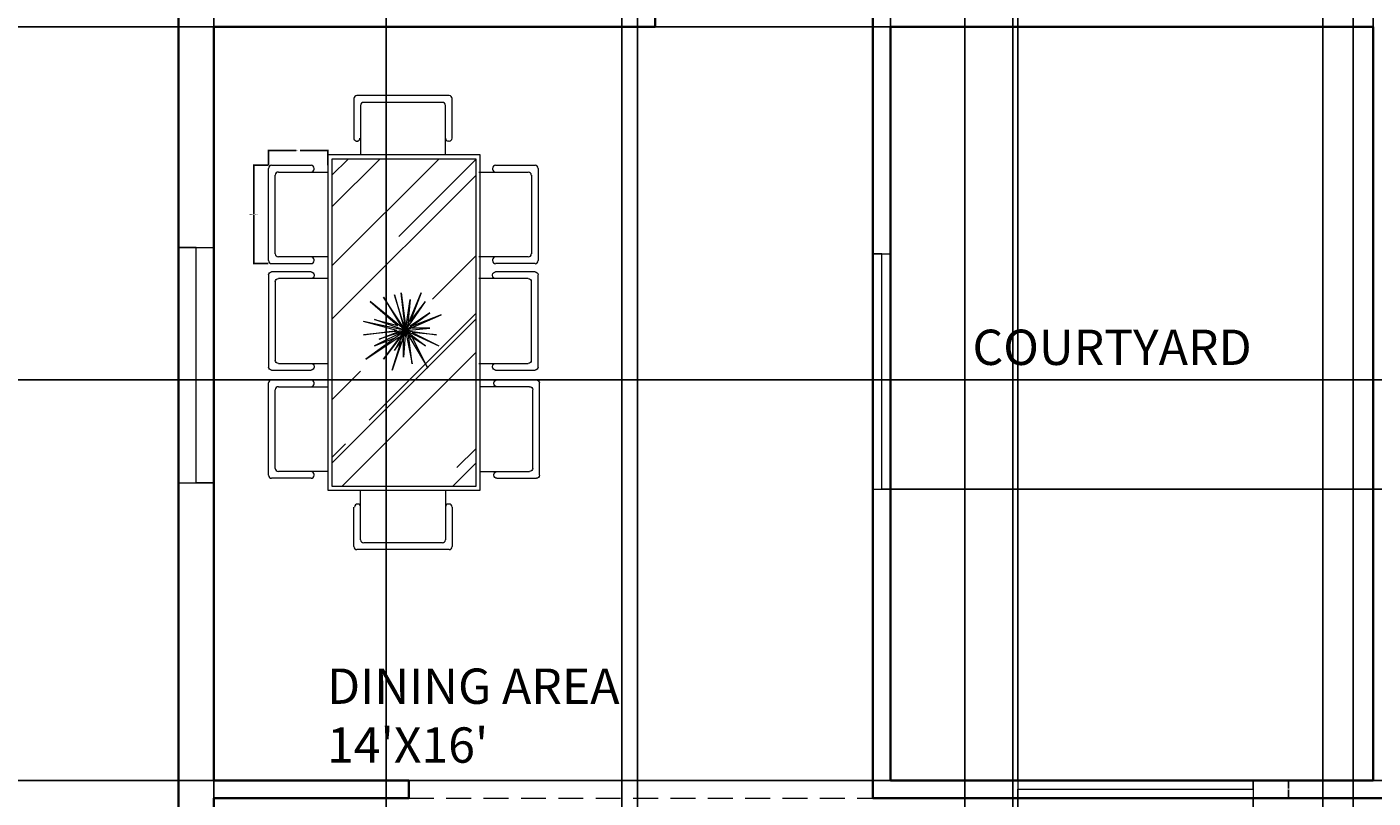
# Model space of a CAD drawing. Units: inches. Extents: x 1770 to 2988, y 1161 to 3221.
# Tile 9 of 44: x 2113 to 2456, y 1835 to 2032. Entities that reach past the tile are written whole.
import ezdxf

# ---------------------------------------------------------------- set-up
doc = ezdxf.new("R2010")
doc.units = ezdxf.units.IN
doc.linetypes.add('DASHED2', pattern=[9.525, 6.35, -3.175])
for name, color, linetype, lineweight in [('A-ANNO-DIMS', 2, 'Continuous', 18), ('A-AREA-IDEN', 7, 'Continuous', 18), ('A-FURN', 8, 'Continuous', 13), ('A-GLAZ', 4, 'Continuous', 18), ('A-WALL', 7, 'Continuous', 35), ('A-WALL-OVHD', 7, 'DASHED2', 18)]:
    doc.layers.add(name, color=color, linetype=linetype, lineweight=lineweight)
doc.styles.get("Standard").update_dxf_attribs({"font": 'arial.ttf'})
doc.dimstyles.get("Standard").update_dxf_attribs({"dimtxt": 0.18, "dimasz": 0.18, "dimexe": 0.18, "dimexo": 0.0625, "dimgap": 0.09, "dimtad": 0, "dimtih": 1, "dimtoh": 1, "dimdec": 4, "dimzin": 0, "dimdsep": 46, "dimtxsty": 'Standard', "dimcen": 0.09, "dimadec": 0, "dimazin": 0, "dimtfac": 1, "dimtdec": 4, "dimtofl": 0, "dimtmove": 0, "dimatfit": 3, "dimfxl": 1, "dimtolj": 1, "dimtzin": 0, "dimarcsym": 0})

# ---------------------------------------------------------------- blocks, each defined once
blk = doc.blocks.new('CHAIR-DINING-SIDE')
for p, q in [((0, 0.78), (0, 24.29)), ((0.78, 25.06), (10.85, 25.06)), ((11.62, 24.11), (11.62, 24.29)), ((1.73, 2.51), (1.73, 22.56)), ((2.51, 23.34), (15.12, 23.34)), ((15.12, 1.73), (2.51, 1.73)), ((11.62, 0.78), (11.62, 0.95)), ((10.85, 0), (0.78, 0))]:
    blk.add_line(p, q)
for centre, start, end in [((0.78, 24.29), 90, 180), ((10.85, 24.29), 0, 90), ((10.85, 24.11), 270, 0), ((2.51, 22.56), 90, 180), ((0.78, 0.78), 180, 270), ((2.51, 2.51), 180, 270), ((10.85, 0.95), 0, 90), ((10.85, 0.78), 270, 0)]:
    blk.add_arc(centre, 0.778, start, end)
blk = doc.blocks.new('WIN-60-EXT')
for p, q in [((0, 9), (0, 0)), ((60, 4.5), (60, 9)), ((60, 9), (60, 0)), ((0, 0), (0, 4.5)), ((0, 4.5), (60, 4.5))]:
    blk.add_line(p, q)
blk = doc.blocks.new('WIN-60-COURTYARD')
for p, q in [((0, 4.5), (0, 0)), ((60, 2.25), (60, 4.5)), ((60, 4.5), (60, 0)), ((0, 0), (0, 2.25)), ((0, 2.25), (60, 2.25))]:
    blk.add_line(p, q)
blk = doc.blocks.new('*D34')
at = {"layer": 'A-ANNO-DIMS', "color": 0, "lineweight": -2, "transparency": 16777216}
for p, q in [((2365.67, 1835.14), (2365.67, 1826.02)), ((2425.67, 1835.14), (2425.67, 1826.02)), ((2365.85, 1826.2), (2394.35, 1826.2)), ((2425.49, 1826.2), (2397, 1826.2))]:
    blk.add_line(p, q, dxfattribs=at)
at = {"layer": 'A-ANNO-DIMS', "color": 0, "transparency": 16777216}
for points in [[(2365.85, 1826.23), (2365.85, 1826.17), (2365.67, 1826.2)], [(2425.49, 1826.23), (2425.49, 1826.17), (2425.67, 1826.2)]]:
    blk.add_solid(points, dxfattribs=at)
at = {"layer": 'Defpoints', "color": 0, "transparency": 16777216}
for p in [(2365.67, 1835.2), (2425.67, 1835.2), (2425.67, 1826.2)]:
    blk.add_point(p, dxfattribs=at)
at = {"layer": 'A-ANNO-DIMS', "color": 0, "transparency": 16777216, "insert": (2395.67, 1826.2), "char_height": 0.18, "attachment_point": 5}
blk.add_mtext('\\A1;COURT WIN. 60 TYP.', dxfattribs=at)
blk = doc.blocks.new('*D35')
at = {"layer": 'A-ANNO-DIMS', "color": 0, "lineweight": -2, "transparency": 16777216}
for p, q in [((2425.73, 1839.7), (2434.85, 1839.7)), ((2434.67, 1839.52), (2434.67, 1837.63)), ((2434.67, 1835.38), (2434.67, 1837.27)), ((2425.73, 1835.2), (2434.85, 1835.2))]:
    blk.add_line(p, q, dxfattribs=at)
at = {"layer": 'A-ANNO-DIMS', "color": 0, "transparency": 16777216}
for points in [[(2434.64, 1839.52), (2434.7, 1839.52), (2434.67, 1839.7)], [(2434.64, 1835.38), (2434.7, 1835.38), (2434.67, 1835.2)]]:
    blk.add_solid(points, dxfattribs=at)
at = {"layer": 'Defpoints', "color": 0, "transparency": 16777216}
for p in [(2425.67, 1839.7), (2434.67, 1839.7), (2425.67, 1835.2)]:
    blk.add_point(p, dxfattribs=at)
at = {"layer": 'A-ANNO-DIMS', "color": 0, "transparency": 16777216, "insert": (2434.67, 1837.45), "char_height": 0.18, "attachment_point": 5}
blk.add_mtext('\\A1;5 TYP.', dxfattribs=at)
blk = doc.blocks.new('*D36')
at = {"layer": 'A-ANNO-DIMS', "color": 0, "lineweight": -2, "transparency": 16777216}
for p, q in [((2174.57, 1996.44), (2170.7, 1996.44)), ((2170.88, 1996.26), (2170.88, 1984.09)), ((2170.88, 1971.56), (2170.88, 1983.73)), ((2174.57, 1971.38), (2170.7, 1971.38))]:
    blk.add_line(p, q, dxfattribs=at)
at = {"layer": 'A-ANNO-DIMS', "color": 0, "transparency": 16777216}
for points in [[(2170.85, 1996.26), (2170.91, 1996.26), (2170.88, 1996.44)], [(2170.85, 1971.56), (2170.91, 1971.56), (2170.88, 1971.38)]]:
    blk.add_solid(points, dxfattribs=at)
at = {"layer": 'Defpoints', "color": 0, "transparency": 16777216}
for p in [(2170.88, 1996.44), (2174.63, 1996.44), (2174.63, 1971.38)]:
    blk.add_point(p, dxfattribs=at)
at = {"layer": 'A-ANNO-DIMS', "color": 0, "transparency": 16777216, "insert": (2170.88, 1983.91), "char_height": 0.18, "attachment_point": 5}
blk.add_mtext('\\A1;SIDE CHAIR 25 TYP.', dxfattribs=at)
blk = doc.blocks.new('*D37')
at = {"layer": 'A-ANNO-DIMS', "color": 0, "lineweight": -2, "transparency": 16777216}
for p, q in [((2174.63, 1996.5), (2174.63, 2000.38)), ((2174.81, 2000.2), (2181.68, 2000.2)), ((2189.57, 2000.2), (2182.71, 2000.2)), ((2189.75, 1996.5), (2189.75, 2000.38))]:
    blk.add_line(p, q, dxfattribs=at)
at = {"layer": 'A-ANNO-DIMS', "color": 0, "transparency": 16777216}
for points in [[(2174.81, 2000.23), (2174.81, 2000.17), (2174.63, 2000.2)], [(2189.57, 2000.23), (2189.57, 2000.17), (2189.75, 2000.2)]]:
    blk.add_solid(points, dxfattribs=at)
at = {"layer": 'Defpoints', "color": 0, "transparency": 16777216}
for p in [(2189.75, 2000.2), (2174.63, 1996.44), (2189.75, 1996.44)]:
    blk.add_point(p, dxfattribs=at)
at = {"layer": 'A-ANNO-DIMS', "color": 0, "transparency": 16777216, "insert": (2182.19, 2000.2), "char_height": 0.18, "attachment_point": 5}
blk.add_mtext('\\A1;15 TYP.', dxfattribs=at)
blk = doc.blocks.new('*D63')
at = {"layer": 'A-ANNO-DIMS', "color": 0, "lineweight": -2, "transparency": 16777216}
for p, q in [((2352.17, 1323.59), (2352.17, 2570.7)), ((2352.35, 2570.52), (2401.24, 2570.52)), ((2450.91, 2570.52), (2402.02, 2570.52)), ((2451.09, 1323.59), (2451.09, 2570.7))]:
    blk.add_line(p, q, dxfattribs=at)
at = {"layer": 'A-ANNO-DIMS', "color": 0, "transparency": 16777216}
for points in [[(2352.35, 2570.55), (2352.35, 2570.49), (2352.17, 2570.52)], [(2450.91, 2570.55), (2450.91, 2570.49), (2451.09, 2570.52)]]:
    blk.add_solid(points, dxfattribs=at)
at = {"layer": 'Defpoints', "color": 0, "transparency": 16777216}
for p in [(2451.09, 2570.52), (2352.17, 1323.53), (2451.09, 1323.53)]:
    blk.add_point(p, dxfattribs=at)
at = {"layer": 'A-ANNO-DIMS', "color": 0, "transparency": 16777216, "insert": (2401.63, 2570.52), "char_height": 0.18, "attachment_point": 5}
blk.add_mtext('\\A1;98.93', dxfattribs=at)
blk = doc.blocks.new('*D68')
at = {"layer": 'A-ANNO-DIMS', "color": 0, "lineweight": -2, "transparency": 16777216}
for p, q in [((2333.2, 2031.76), (2333.2, 2570.7)), ((2333.38, 2570.52), (2394.42, 2570.52)), ((2456.02, 2570.52), (2394.98, 2570.52)), ((2456.2, 2031.76), (2456.2, 2570.7))]:
    blk.add_line(p, q, dxfattribs=at)
at = {"layer": 'A-ANNO-DIMS', "color": 0, "transparency": 16777216}
for points in [[(2333.38, 2570.55), (2333.38, 2570.49), (2333.2, 2570.52)], [(2456.02, 2570.55), (2456.02, 2570.49), (2456.2, 2570.52)]]:
    blk.add_solid(points, dxfattribs=at)
at = {"layer": 'Defpoints', "color": 0, "transparency": 16777216}
for p in [(2456.2, 2570.52), (2333.2, 2031.7), (2456.2, 2031.7)]:
    blk.add_point(p, dxfattribs=at)
at = {"layer": 'A-ANNO-DIMS', "color": 0, "transparency": 16777216, "insert": (2394.7, 2570.52), "char_height": 0.18, "attachment_point": 5}
blk.add_mtext('\\A1;123', dxfattribs=at)
blk = doc.blocks.new('*D69')
at = {"layer": 'A-ANNO-DIMS', "color": 0, "lineweight": -2, "transparency": 16777216}
for p, q in [((2333.13, 2031.7), (1907.1, 2031.7)), ((1907.28, 2031.52), (1907.28, 1935.88)), ((1907.28, 1839.88), (1907.28, 1935.52)), ((2333.13, 1839.7), (1907.1, 1839.7))]:
    blk.add_line(p, q, dxfattribs=at)
at = {"layer": 'A-ANNO-DIMS', "color": 0, "transparency": 16777216}
for points in [[(1907.25, 2031.52), (1907.31, 2031.52), (1907.28, 2031.7)], [(1907.25, 1839.88), (1907.31, 1839.88), (1907.28, 1839.7)]]:
    blk.add_solid(points, dxfattribs=at)
at = {"layer": 'Defpoints', "color": 0, "transparency": 16777216}
for p in [(1907.28, 2031.7), (2333.2, 2031.7), (2333.2, 1839.7)]:
    blk.add_point(p, dxfattribs=at)
at = {"layer": 'A-ANNO-DIMS', "color": 0, "transparency": 16777216, "insert": (1907.28, 1935.7), "char_height": 0.18, "attachment_point": 5}
blk.add_mtext('\\A1;192', dxfattribs=at)
blk = doc.blocks.new('*D70')
at = {"layer": 'A-ANNO-DIMS', "color": 0, "lineweight": -2, "transparency": 16777216}
for p, q in [((2160.7, 2171.14), (2160.7, 1165.57)), ((2268.7, 2171.14), (2268.7, 1165.57)), ((2160.88, 1165.75), (2214.42, 1165.75)), ((2268.52, 1165.75), (2214.98, 1165.75))]:
    blk.add_line(p, q, dxfattribs=at)
at = {"layer": 'A-ANNO-DIMS', "color": 0, "transparency": 16777216}
for points in [[(2160.88, 1165.78), (2160.88, 1165.72), (2160.7, 1165.75)], [(2268.52, 1165.78), (2268.52, 1165.72), (2268.7, 1165.75)]]:
    blk.add_solid(points, dxfattribs=at)
at = {"layer": 'Defpoints', "color": 0, "transparency": 16777216}
for p in [(2160.7, 2171.2), (2268.7, 2171.2), (2268.7, 1165.75)]:
    blk.add_point(p, dxfattribs=at)
at = {"layer": 'A-ANNO-DIMS', "color": 0, "transparency": 16777216, "insert": (2214.7, 1165.75), "char_height": 0.18, "attachment_point": 5}
blk.add_mtext('\\A1;108', dxfattribs=at)
blk = doc.blocks.new('*D79')
at = {"layer": 'A-ANNO-DIMS', "color": 0, "lineweight": -2, "transparency": 16777216}
for p, q in [((2151.7, 1610.26), (2151.7, 2570.7)), ((2151.88, 2570.52), (2177.78, 2570.52)), ((2204.48, 2570.52), (2178.57, 2570.52)), ((2204.66, 1610.26), (2204.66, 2570.7))]:
    blk.add_line(p, q, dxfattribs=at)
at = {"layer": 'A-ANNO-DIMS', "color": 0, "transparency": 16777216}
for points in [[(2151.88, 2570.55), (2151.88, 2570.49), (2151.7, 2570.52)], [(2204.48, 2570.55), (2204.48, 2570.49), (2204.66, 2570.52)]]:
    blk.add_solid(points, dxfattribs=at)
at = {"layer": 'Defpoints', "color": 0, "transparency": 16777216}
for p in [(2204.66, 2570.52), (2151.7, 1610.2), (2204.66, 1610.2)]:
    blk.add_point(p, dxfattribs=at)
at = {"layer": 'A-ANNO-DIMS', "color": 0, "transparency": 16777216, "insert": (2178.18, 2570.52), "char_height": 0.18, "attachment_point": 5}
blk.add_mtext('\\A1;52.96', dxfattribs=at)
blk = doc.blocks.new('*D80')
at = {"layer": 'A-ANNO-DIMS', "color": 0, "lineweight": -2, "transparency": 16777216}
for p, q in [((2264.66, 1610.26), (2264.66, 2570.7)), ((2264.84, 2570.52), (2314.14, 2570.52)), ((2364.23, 2570.52), (2314.93, 2570.52)), ((2364.41, 1610.26), (2364.41, 2570.7))]:
    blk.add_line(p, q, dxfattribs=at)
at = {"layer": 'A-ANNO-DIMS', "color": 0, "transparency": 16777216}
for points in [[(2264.84, 2570.55), (2264.84, 2570.49), (2264.66, 2570.52)], [(2364.23, 2570.55), (2364.23, 2570.49), (2364.41, 2570.52)]]:
    blk.add_solid(points, dxfattribs=at)
at = {"layer": 'Defpoints', "color": 0, "transparency": 16777216}
for p in [(2364.41, 2570.52), (2264.66, 1610.2), (2364.41, 1610.2)]:
    blk.add_point(p, dxfattribs=at)
at = {"layer": 'A-ANNO-DIMS', "color": 0, "transparency": 16777216, "insert": (2314.53, 2570.52), "char_height": 0.18, "attachment_point": 5}
blk.add_mtext('\\A1;99.76', dxfattribs=at)
blk = doc.blocks.new('*D81')
at = {"layer": 'A-ANNO-DIMS', "color": 0, "lineweight": -2, "transparency": 16777216}
for p, q in [((2364.41, 1610.26), (2364.41, 2570.7)), ((2364.59, 2570.52), (2403.51, 2570.52)), ((2443.21, 2570.52), (2404.29, 2570.52)), ((2443.39, 1610.26), (2443.39, 2570.7))]:
    blk.add_line(p, q, dxfattribs=at)
at = {"layer": 'A-ANNO-DIMS', "color": 0, "transparency": 16777216}
for points in [[(2364.59, 2570.55), (2364.59, 2570.49), (2364.41, 2570.52)], [(2443.21, 2570.55), (2443.21, 2570.49), (2443.39, 2570.52)]]:
    blk.add_solid(points, dxfattribs=at)
at = {"layer": 'Defpoints', "color": 0, "transparency": 16777216}
for p in [(2443.39, 2570.52), (2364.41, 1610.2), (2443.39, 1610.2)]:
    blk.add_point(p, dxfattribs=at)
at = {"layer": 'A-ANNO-DIMS', "color": 0, "transparency": 16777216, "insert": (2403.9, 2570.52), "char_height": 0.18, "attachment_point": 5}
blk.add_mtext('\\A1;78.97', dxfattribs=at)
blk = doc.blocks.new('*D82')
at = {"layer": 'A-ANNO-DIMS', "color": 0, "lineweight": -2, "transparency": 16777216}
for p, q in [((2443.39, 1610.26), (2443.39, 2570.7)), ((2443.57, 2570.52), (2486.45, 2570.52)), ((2530.12, 2570.52), (2487.24, 2570.52)), ((2530.3, 1610.26), (2530.3, 2570.7))]:
    blk.add_line(p, q, dxfattribs=at)
at = {"layer": 'A-ANNO-DIMS', "color": 0, "transparency": 16777216}
for points in [[(2443.57, 2570.55), (2443.57, 2570.49), (2443.39, 2570.52)], [(2530.12, 2570.55), (2530.12, 2570.49), (2530.3, 2570.52)]]:
    blk.add_solid(points, dxfattribs=at)
at = {"layer": 'Defpoints', "color": 0, "transparency": 16777216}
for p in [(2530.3, 2570.52), (2443.39, 1610.2), (2530.3, 1610.2)]:
    blk.add_point(p, dxfattribs=at)
at = {"layer": 'A-ANNO-DIMS', "color": 0, "transparency": 16777216, "insert": (2486.85, 2570.52), "char_height": 0.18, "attachment_point": 5}
blk.add_mtext('\\A1;86.92', dxfattribs=at)
blk = doc.blocks.new('*D90')
at = {"layer": 'A-ANNO-DIMS', "color": 0, "lineweight": -2, "transparency": 16777216}
for p, q in [((2616.63, 1941.8), (1907.1, 1941.8)), ((1907.28, 1941.62), (1907.28, 1890.93)), ((1907.28, 1839.88), (1907.28, 1890.57)), ((2616.63, 1839.7), (1907.1, 1839.7))]:
    blk.add_line(p, q, dxfattribs=at)
at = {"layer": 'A-ANNO-DIMS', "color": 0, "transparency": 16777216}
for points in [[(1907.25, 1941.62), (1907.31, 1941.62), (1907.28, 1941.8)], [(1907.25, 1839.88), (1907.31, 1839.88), (1907.28, 1839.7)]]:
    blk.add_solid(points, dxfattribs=at)
at = {"layer": 'Defpoints', "color": 0, "transparency": 16777216}
for p in [(1907.28, 1941.8), (2616.7, 1941.8), (2616.7, 1839.7)]:
    blk.add_point(p, dxfattribs=at)
at = {"layer": 'A-ANNO-DIMS', "color": 0, "transparency": 16777216, "insert": (1907.28, 1890.75), "char_height": 0.18, "attachment_point": 5}
blk.add_mtext('\\A1;102.1', dxfattribs=at)
blk = doc.blocks.new('*D91')
at = {"layer": 'A-ANNO-DIMS', "color": 0, "lineweight": -2, "transparency": 16777216}
for p, q in [((2333.2, 1839.76), (2333.2, 2570.7)), ((2333.38, 2570.52), (2348.97, 2570.52)), ((2365.49, 2570.52), (2349.9, 2570.52)), ((2365.67, 1839.76), (2365.67, 2570.7))]:
    blk.add_line(p, q, dxfattribs=at)
at = {"layer": 'A-ANNO-DIMS', "color": 0, "transparency": 16777216}
for points in [[(2333.38, 2570.55), (2333.38, 2570.49), (2333.2, 2570.52)], [(2365.49, 2570.55), (2365.49, 2570.49), (2365.67, 2570.52)]]:
    blk.add_solid(points, dxfattribs=at)
at = {"layer": 'Defpoints', "color": 0, "transparency": 16777216}
for p in [(2365.67, 2570.52), (2333.2, 1839.7), (2365.67, 1839.7)]:
    blk.add_point(p, dxfattribs=at)
at = {"layer": 'A-ANNO-DIMS', "color": 0, "transparency": 16777216, "insert": (2349.43, 2570.52), "char_height": 0.18, "attachment_point": 5}
blk.add_mtext('\\A1;32.476', dxfattribs=at)
blk = doc.blocks.new('*D92')
at = {"layer": 'A-ANNO-DIMS', "color": 0, "lineweight": -2, "transparency": 16777216}
for p, q in [((2333.26, 1913.9), (2866.87, 1913.9)), ((2866.69, 1913.72), (2866.69, 1876.98)), ((2866.69, 1839.88), (2866.69, 1876.62)), ((2333.26, 1839.7), (2866.87, 1839.7))]:
    blk.add_line(p, q, dxfattribs=at)
at = {"layer": 'A-ANNO-DIMS', "color": 0, "transparency": 16777216}
for points in [[(2866.66, 1913.72), (2866.72, 1913.72), (2866.69, 1913.9)], [(2866.66, 1839.88), (2866.72, 1839.88), (2866.69, 1839.7)]]:
    blk.add_solid(points, dxfattribs=at)
at = {"layer": 'Defpoints', "color": 0, "transparency": 16777216}
for p in [(2333.2, 1913.9), (2866.69, 1913.9), (2333.2, 1839.7)]:
    blk.add_point(p, dxfattribs=at)
at = {"layer": 'A-ANNO-DIMS', "color": 0, "transparency": 16777216, "insert": (2866.69, 1876.8), "char_height": 0.18, "attachment_point": 5}
blk.add_mtext('\\A1;74.2', dxfattribs=at)

msp = doc.modelspace()

# ---------------------------------------------------------------- linework, layer by layer
at = {"layer": 'A-FURN'}
for p, q in [((2196.3997, 2013.4311), (2196.3997, 2003.3617)), ((2220.6858, 2014.2089), (2197.1775, 2014.2089)), ((2198.1282, 2011.7025), (2198.1282, 1999.0887)), ((2218.9573, 2012.4804), (2198.9061, 2012.4804)), ((2219.7351, 1999.0887), (2219.7351, 2011.7025)), ((2221.4637, 2003.3617), (2221.4637, 2013.4311)), ((2197.3504, 2002.5839), (2197.1775, 2002.5839)), ((2220.6858, 2002.5839), (2220.513, 2002.5839)), ((2228.6216, 1999.0887), (2189.7291, 1999.0887)), ((2189.7291, 1999.0887), (2189.7291, 1913.6213)), ((2190.8095, 1970.7936), (2218.0242, 1998.0083)), ((2190.8095, 1985.8276), (2202.9902, 1998.0083)), ((2227.5412, 1998.0083), (2190.8095, 1998.0083)), ((2190.8095, 1998.0083), (2190.8095, 1914.7017)), ((2190.8095, 1993.8946), (2194.9232, 1998.0083)), ((2207.8148, 1978.2653), (2227.5412, 1997.9917)), ((2227.5412, 1914.7017), (2227.5412, 1998.0083)), ((2228.6216, 1913.6213), (2228.6216, 1999.0887)), ((2190.8095, 1957.2264), (2227.5412, 1993.9582)), ((2216.4318, 1962.3146), (2227.5412, 1973.424)), ((2203.9343, 1962.832), (2208.4512, 1955.4922)), ((2209.5804, 1954.363), (2203.9343, 1962.832)), ((2206.7573, 1963.3966), (2209.0158, 1955.4922)), ((2209.5804, 1954.363), (2206.7573, 1963.3966)), ((2208.4512, 1963.9612), (2209.5804, 1955.4922)), ((2209.5804, 1954.363), (2208.4512, 1963.9612)), ((2209.5804, 1954.363), (2213.5326, 1963.9612)), ((2213.5326, 1963.9612), (2210.7096, 1956.6214)), ((2200.5467, 1961.7028), (2207.5801, 1955.6119)), ((2209.5804, 1954.363), (2200.5467, 1961.7028)), ((2209.5804, 1954.363), (2210.7096, 1962.2674)), ((2209.5804, 1954.363), (2214.6618, 1961.7028)), ((2210.7096, 1962.2674), (2210.145, 1956.0568)), ((2210.7096, 1956.6214), (2214.6618, 1961.7028)), ((2190.8095, 1920.5583), (2227.5412, 1957.29)), ((2207.3219, 1954.363), (2198.8529, 1956.6214)), ((2209.5804, 1954.363), (2198.8529, 1956.6214)), ((2200.2978, 1931.5134), (2227.5412, 1958.7567)), ((2201.6759, 1957.186), (2207.5801, 1955.6119)), ((2209.5804, 1954.363), (2201.6759, 1957.186)), ((2209.5804, 1954.363), (2215.791, 1958.8798)), ((2209.5804, 1954.363), (2218.614, 1958.3152)), ((2215.791, 1958.8798), (2210.7096, 1955.4922)), ((2218.614, 1958.3152), (2211.2742, 1955.4922)), ((2198.8529, 1953.2338), (2207.3219, 1954.363)), ((2209.5804, 1954.363), (2198.8529, 1953.2338)), ((2209.5804, 1954.363), (2199.4175, 1947.0232)), ((2199.4175, 1947.0232), (2207.8866, 1952.6692)), ((2209.5804, 1954.363), (2201.6759, 1950.4108)), ((2201.6759, 1950.4108), (2207.1273, 1952.5913)), ((2209.5804, 1954.363), (2202.8051, 1952.1046)), ((2202.8051, 1952.1046), (2208.0479, 1954.2017)), ((2209.5804, 1954.363), (2203.9343, 1947.0232)), ((2203.9343, 1947.0232), (2209.0158, 1953.7984)), ((2209.5804, 1954.363), (2206.1927, 1944.2002)), ((2209.5804, 1954.363), (2206.7573, 1949.2816)), ((2209.5804, 1954.363), (2209.0158, 1947.5878)), ((2209.0158, 1947.5878), (2209.0158, 1952.6692)), ((2209.5804, 1954.363), (2215.791, 1954.9276)), ((2209.5804, 1954.363), (2217.4848, 1953.2338)), ((2209.5804, 1954.363), (2214.6618, 1950.4108)), ((2209.5804, 1954.363), (2218.0494, 1950.4108)), ((2209.5804, 1954.363), (2215.2264, 1944.7648)), ((2209.5804, 1954.363), (2211.2742, 1945.894)), ((2214.6618, 1950.4108), (2210.3025, 1953.1353)), ((2211.2742, 1945.894), (2210.3025, 1953.1353)), ((2215.791, 1954.9276), (2211.2742, 1954.9276)), ((2211.2742, 1953.7984), (2218.0494, 1950.4108)), ((2217.4848, 1953.2338), (2211.2742, 1953.7984)), ((2206.1927, 1944.2002), (2208.4512, 1951.54)), ((2206.7573, 1949.2816), (2208.4512, 1951.54)), ((2215.2264, 1944.7648), (2211.3768, 1952.4639)), ((2218.0494, 1950.4108), (2218.0494, 1950.4108)), ((2193.3865, 1914.7017), (2227.5412, 1948.8563)), ((2190.8095, 1936.6923), (2198.0977, 1943.9805)), ((2190.8095, 1922.025), (2194.2476, 1925.4631)), ((2222.6654, 1919.4129), (2227.5412, 1924.2887)), ((2221.621, 1914.7017), (2227.5412, 1920.6219)), ((2189.7291, 1913.6213), (2228.6216, 1913.6213)), ((2190.8095, 1914.7017), (2227.5412, 1914.7017)), ((2198.1282, 1901.0075), (2198.1282, 1913.6213)), ((2219.7351, 1913.6213), (2219.7351, 1901.0075)), ((2196.3997, 1899.2789), (2196.3997, 1909.3483)), ((2197.3504, 1910.1261), (2197.1775, 1910.1261)), ((2220.6858, 1910.1261), (2220.513, 1910.1261)), ((2221.4637, 1909.3483), (2221.4637, 1899.2789)), ((2220.6858, 1898.5011), (2197.1775, 1898.5011)), ((2218.9573, 1900.2296), (2198.9061, 1900.2296))]:
    msp.add_line(p, q, dxfattribs=at)
for centre, start, end in [((2197.1775, 2013.4311), 90, 180), ((2198.9061, 2011.7025), 90, 180), ((2218.9573, 2011.7025), 0, 90), ((2220.6858, 2013.4311), 0, 90), ((2197.1775, 2003.3617), 180, 0.058348), ((2220.513, 2003.3617), 180, 270), ((2220.6858, 2003.3617), 270, 0), ((2197.3504, 1909.3483), 0, 179.863122), ((2220.513, 1909.3483), 90, 180), ((2220.6858, 1909.3483), 0, 90), ((2198.9061, 1901.0075), 180, 270), ((2218.9573, 1901.0075), 270, 0), ((2197.1775, 1899.2789), 180, 270), ((2220.6858, 1899.2789), 270, 0)]:
    msp.add_arc(centre, 0.7778, start, end, dxfattribs=at)
at = {"layer": 'A-WALL'}
for p, q in [((2151.696, 2376.7021), (2151.696, 1610.2021)), ((2273.196, 2171.2021), (2273.196, 2031.7021)), ((2328.696, 2036.2021), (2328.696, 1835.2021)), ((2160.696, 2031.7021), (2273.196, 2031.7021)), ((2160.696, 2031.7021), (2160.696, 1839.7021)), ((2333.196, 2031.7021), (2333.196, 1839.7021)), ((2333.196, 2031.7021), (2456.196, 2031.7021)), ((2456.196, 2031.7021), (2456.196, 1839.7021)), ((2160.696, 1839.7021), (2210.4281, 1839.7021)), ((2210.4281, 1839.7021), (2210.4281, 1835.2021)), ((2333.196, 1839.7021), (2456.196, 1839.7021)), ((2160.696, 1835.2021), (2210.4281, 1835.2021)), ((2160.696, 1835.2021), (2160.696, 1619.2021)), ((2328.696, 1835.2021), (2464.9215, 1835.2021))]:
    msp.add_line(p, q, dxfattribs=at)
at = {"layer": 'A-WALL-OVHD'}
for p, q in [((2273.196, 2031.7021), (2328.696, 2031.7021)), ((2210.4281, 1839.7021), (2328.696, 1839.7021)), ((2210.4281, 1835.2021), (2328.696, 1835.2021))]:
    msp.add_line(p, q, dxfattribs=at)

# ---------------------------------------------------------------- block references
at = {"layer": 'A-FURN'}
for p in [(2174.635, 1971.377), (2174.635, 1916.687)]:
    msp.add_blockref('CHAIR-DINING-SIDE', p, dxfattribs=at)
at = {"layer": 'A-FURN', "rotation": 180}
msp.add_blockref('CHAIR-DINING-SIDE', (2243.3634, 1996.4402), dxfattribs=at)
at = {"layer": 'A-FURN', "extrusion": (0, 0, -1), "zscale": -1, "rotation": 180}
msp.add_blockref('CHAIR-DINING-SIDE', (-2174.635, 1969.3044), dxfattribs=at)
at = {"layer": 'A-FURN', "extrusion": (0, 0, -1), "zscale": -1}
for p in [(-2243.3634, 1944.2412), (-2243.7157, 1916.687)]:
    msp.add_blockref('CHAIR-DINING-SIDE', p, dxfattribs=at)
at = {"layer": 'A-GLAZ', "rotation": 90}
for name, p in [('WIN-60-EXT', (2160.6961, 1915.5016)), ('WIN-60-COURTYARD', (2333.1961, 1913.8992))]:
    msp.add_blockref(name, p, dxfattribs=at)
at = {"layer": 'A-GLAZ'}
msp.add_blockref('WIN-60-COURTYARD', (2365.672, 1835.202), dxfattribs=at)

# ---------------------------------------------------------------- texts
at = {"layer": 'A-AREA-IDEN', "char_height": 9, "attachment_point": 1}
for s, width, insert in [('COURTYARD', 69.498469, (2354.0805, 1954.5684)), ("DINING AREA\\P14'X16'", 92.538112, (2189.5487, 1868.2134))]:
    msp.add_mtext_dynamic_manual_height_columns(s, width=width, gutter_width=12.5, heights=[0], dxfattribs=dict(at, insert=insert))

# ---------------------------------------------------------------- dimensions: what is measured, and where the dimension line sits
at = {"layer": 'A-ANNO-DIMS'}
for base, p1, p2, override, picture, middle in [((2204.6568, 2570.5247), (2151.696, 1610.2021), (2204.6568, 1610.2021), {"dimdec": 2, "dimlfac": 1, "dimrnd": 0, "dimzin": 0, "dimdsep": 46, "dimlunit": 2}, '*D79', (2178.1764, 2570.5247)), ((2364.4122, 2570.5247), (2264.6568, 1610.2021), (2364.4122, 1610.2021), {"dimdec": 2, "dimlfac": 1, "dimrnd": 0, "dimzin": 0, "dimdsep": 46, "dimlunit": 2}, '*D80', (2314.5345, 2570.5247)), ((2456.196, 2570.5247), (2333.196, 2031.7021), (2456.196, 2031.7021), {"dimdec": 0, "dimlfac": 1, "dimrnd": 0, "dimzin": 0, "dimdsep": 46, "dimlunit": 2}, '*D68', (2394.696, 2570.5247)), ((2365.672, 2570.5247), (2333.196, 1839.7021), (2365.672, 1839.7021), {"dimdec": 3, "dimlfac": 1, "dimrnd": 0, "dimzin": 0, "dimdsep": 46, "dimlunit": 2}, '*D91', (2349.434, 2570.5247)), ((2451.0947, 2570.5247), (2352.1672, 1323.5288), (2451.0947, 1323.5288), {"dimdec": 2, "dimlfac": 1, "dimrnd": 0, "dimzin": 0, "dimdsep": 46, "dimlunit": 2}, '*D63', (2401.631, 2570.5247)), ((2443.3863, 2570.5247), (2364.4122, 1610.2021), (2443.3863, 1610.2021), {"dimdec": 2, "dimlfac": 1, "dimrnd": 0, "dimzin": 0, "dimdsep": 46, "dimlunit": 2}, '*D81', (2403.8993, 2570.5247)), ((2530.3038, 2570.5247), (2443.3863, 1610.2021), (2530.3038, 1610.2021), {"dimdec": 2, "dimlfac": 1, "dimrnd": 0, "dimzin": 0, "dimdsep": 46, "dimlunit": 2}, '*D82', (2486.8451, 2570.5247)), ((2268.696, 1165.752), (2160.696, 2171.2021), (2268.696, 2171.2021), {"dimdec": 0, "dimlfac": 1, "dimrnd": 0, "dimzin": 0, "dimdsep": 46, "dimlunit": 2}, '*D70', (2214.696, 1165.752))]:
    dim = msp.add_linear_dim(base=base, p1=p1, p2=p2, dimstyle='Standard', override=override, dxfattribs=at)
    dim.commit()
    dim.dimension.update_dxf_attribs({"geometry": picture, "text_midpoint": middle})
for base, p1, p2, override, picture, middle in [((1907.2844, 2031.7021), (2333.196, 1839.7021), (2333.196, 2031.7021), {"dimdec": 0, "dimlfac": 1, "dimrnd": 0, "dimzin": 0, "dimdsep": 46, "dimlunit": 2}, '*D69', (1907.2844, 1935.7021)), ((1907.2844, 1941.8004), (2616.696, 1839.7021), (2616.696, 1941.8004), {"dimdec": 1, "dimlfac": 1, "dimrnd": 0, "dimzin": 0, "dimdsep": 46, "dimlunit": 2}, '*D90', (1907.2844, 1890.7512)), ((2866.6874, 1913.8992), (2333.196, 1839.7021), (2333.196, 1913.8992), {"dimdec": 1, "dimlfac": 1, "dimrnd": 0, "dimzin": 0, "dimdsep": 46, "dimlunit": 2}, '*D92', (2866.6874, 1876.8007))]:
    dim = msp.add_linear_dim(base=base, p1=p1, p2=p2, angle=90, dimstyle='Standard', override=override, dxfattribs=at)
    dim.commit()
    dim.dimension.update_dxf_attribs({"geometry": picture, "text_midpoint": middle})
for base, p1, p2, text, picture, middle in [((2189.7549, 2000.2002), (2174.6346, 1996.4406), (2189.7549, 1996.4406), '<> TYP.', '*D37', (2182.1948, 2000.2002)), ((2425.672, 1826.2021), (2365.672, 1835.2021), (2425.672, 1835.2021), 'COURT WIN. <> TYP.', '*D34', (2395.672, 1826.2021))]:
    dim = msp.add_linear_dim(base=base, p1=p1, p2=p2, text=text, dimstyle='Standard', override={"dimdec": 0, "dimlfac": 1, "dimrnd": 0, "dimzin": 0, "dimdsep": 46, "dimlunit": 2}, dxfattribs=at)
    dim.commit()
    dim.dimension.update_dxf_attribs({"geometry": picture, "text_midpoint": middle})
for base, p1, p2, text, picture, middle in [((2170.875, 1996.4406), (2174.6346, 1971.3766), (2174.6346, 1996.4406), 'SIDE CHAIR <> TYP.', '*D36', (2170.875, 1983.9086)), ((2434.6720024489, 1839.7021160144), (2425.6720024489, 1835.2021160144), (2425.6720024489, 1839.7021160144), '<> TYP.', '*D35', (2434.6720024489, 1837.4521160144))]:
    dim = msp.add_linear_dim(base=base, p1=p1, p2=p2, angle=90, text=text, dimstyle='Standard', override={"dimdec": 0, "dimlfac": 1, "dimrnd": 0, "dimzin": 0, "dimdsep": 46, "dimlunit": 2}, dxfattribs=at)
    dim.commit()
    dim.dimension.update_dxf_attribs({"geometry": picture, "text_midpoint": middle})

doc.saveas('drawing.dxf')
